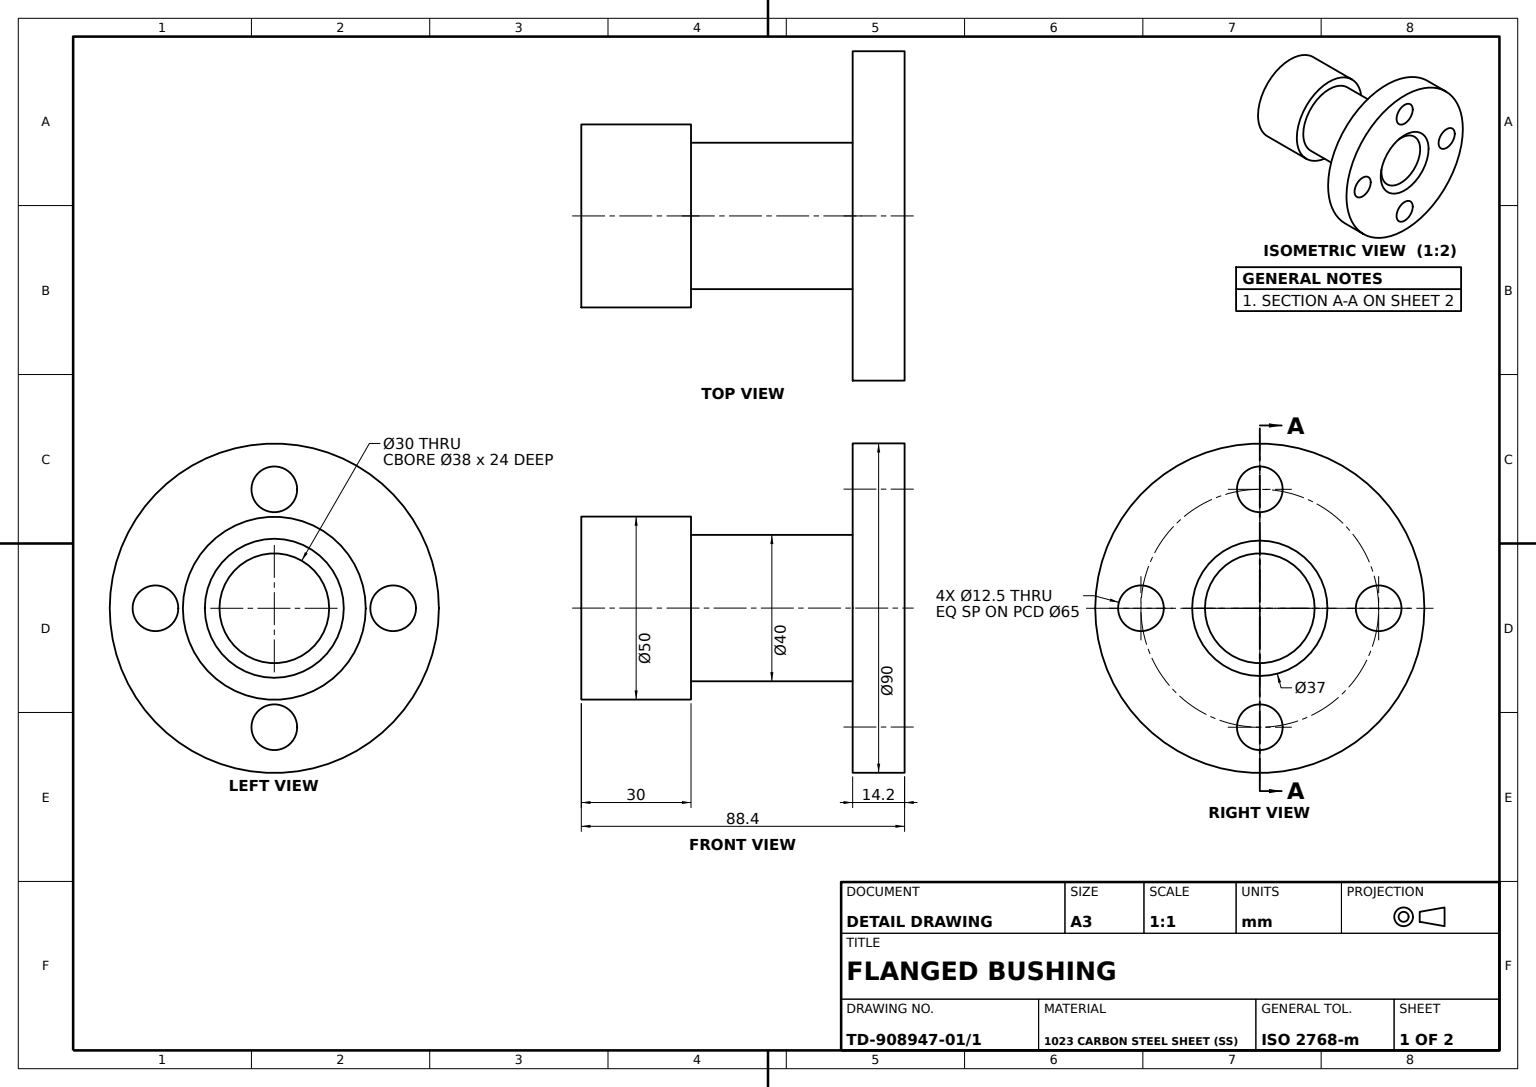
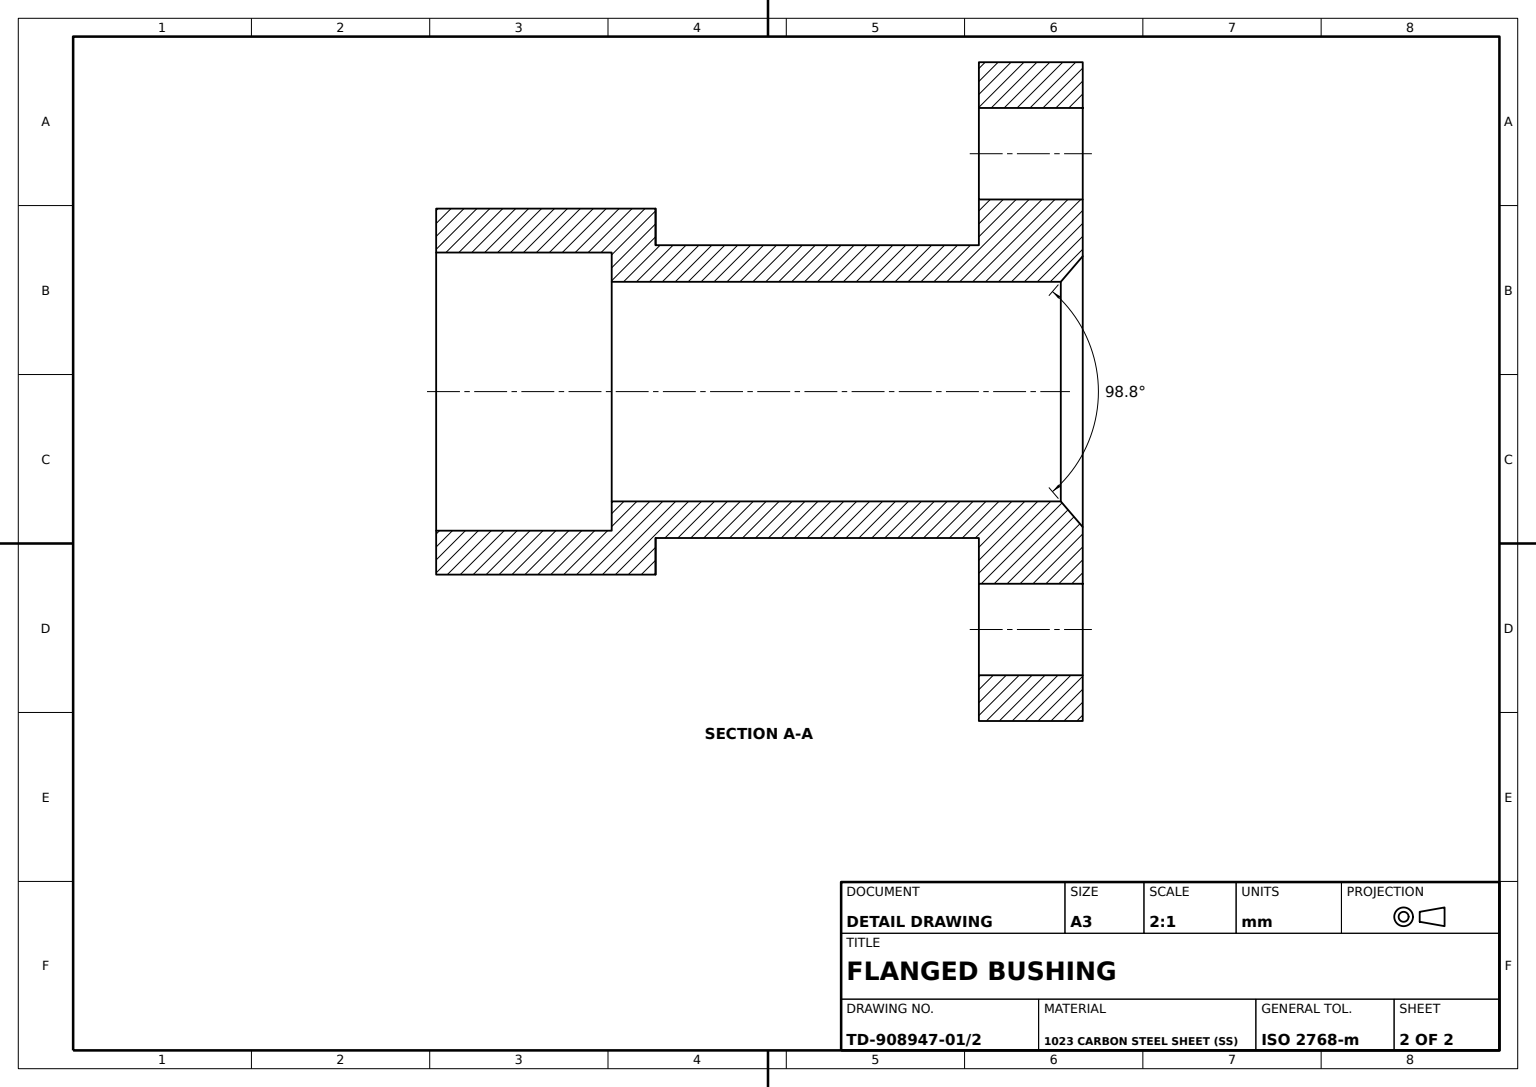
SolidWorks part; units mm, degrees
material "1023 Carbon Steel Sheet (SS)"
ref_plane "Front Plane" through (0, 0, 0) normal (0, 0, 1) x (1, 0, 0)
ref_plane "Top Plane" through (0, 0, 0) normal (0, 1, 0) x (1, 0, 0)
ref_plane "Right Plane" through (0, 0, 0) normal (1, 0, 0) x (0, 0, -1)
sketch "Flange Sketch" plane through (0, 0, 0) normal (0, 0, 1) x (1, 0, 0)
  circle A0 centre (0, 0) radius 15
  circle A1 centre (0, 0) radius 45
  dimension "D1" = 30
  dimension "D2" = 90
extrude "Flange Ø90" add sketch "Flange Sketch" along normal blind 14.2
sketch "Hub Sketch" plane through (0, 0, 14.2) normal (0, 0, 1) x (1, 0, 0)
  circle A0 centre (0, 0) radius 15
  circle A1 centre (0, 0) radius 20
  dimension "D1" = 30
  dimension "D2" = 40
extrude "Hub Ø40" add sketch "Hub Sketch" along normal blind 44.2
sketch "Collar Sketch" plane through (0, 0, 58.4) normal (0, 0, 1) x (1, 0, 0)
  circle A0 centre (0, 0) radius 15
  circle A1 centre (0, 0) radius 25
  dimension "D1" = 30
  dimension "D2" = 50
extrude "Collar Ø50" add sketch "Collar Sketch" along normal blind 6
sketch "End Sleeve Sketch" plane through (0, 0, 64.4) normal (0, 0, 1) x (1, 0, 0)
  circle A0 centre (0, 0) radius 19
  circle A1 centre (0, 0) radius 25
  dimension "D1" = 38
  dimension "D2" = 50
extrude "End Sleeve Ø50 Bore Ø38" add sketch "End Sleeve Sketch" along normal blind 24
fillet "Flange Edge Chamfer" radius 3 1 edges at (15, 0, 0) profile chamfer
sketch "Bolt Holes Set A Sketch" plane through (0, 0, 0) normal (0, 0, 1) x (1, 0, 0)
  line L0 (0, 32.5) -> (0, -32.5)
  circle A0 centre (0, 32.5) radius 6.25
  circle A1 centre (0, -32.5) radius 6.25
  dimension "D3" = 12.5
  dimension "D4" = 12.5
  dimension "D1" = 65
  dimension "D2" = 32.5
extrude "Bolt Holes Set A" cut sketch "Bolt Holes Set A Sketch" along normal blind 24
sketch "Bolt Holes Set B Sketch" plane through (0, 0, 0) normal (0, 0, 1) x (1, 0, 0)
  line L0 (-32.5, 0) -> (32.5, 0)
  circle A0 centre (-32.5, 0) radius 6.25
  circle A1 centre (32.5, 0) radius 6.25
  dimension "D1" = 12.5
  dimension "D2" = 12.5
  dimension "D3" = 65
  dimension "D4" = 32.5
extrude "Bolt Holes Set B" cut sketch "Bolt Holes Set B Sketch" along normal blind 24
